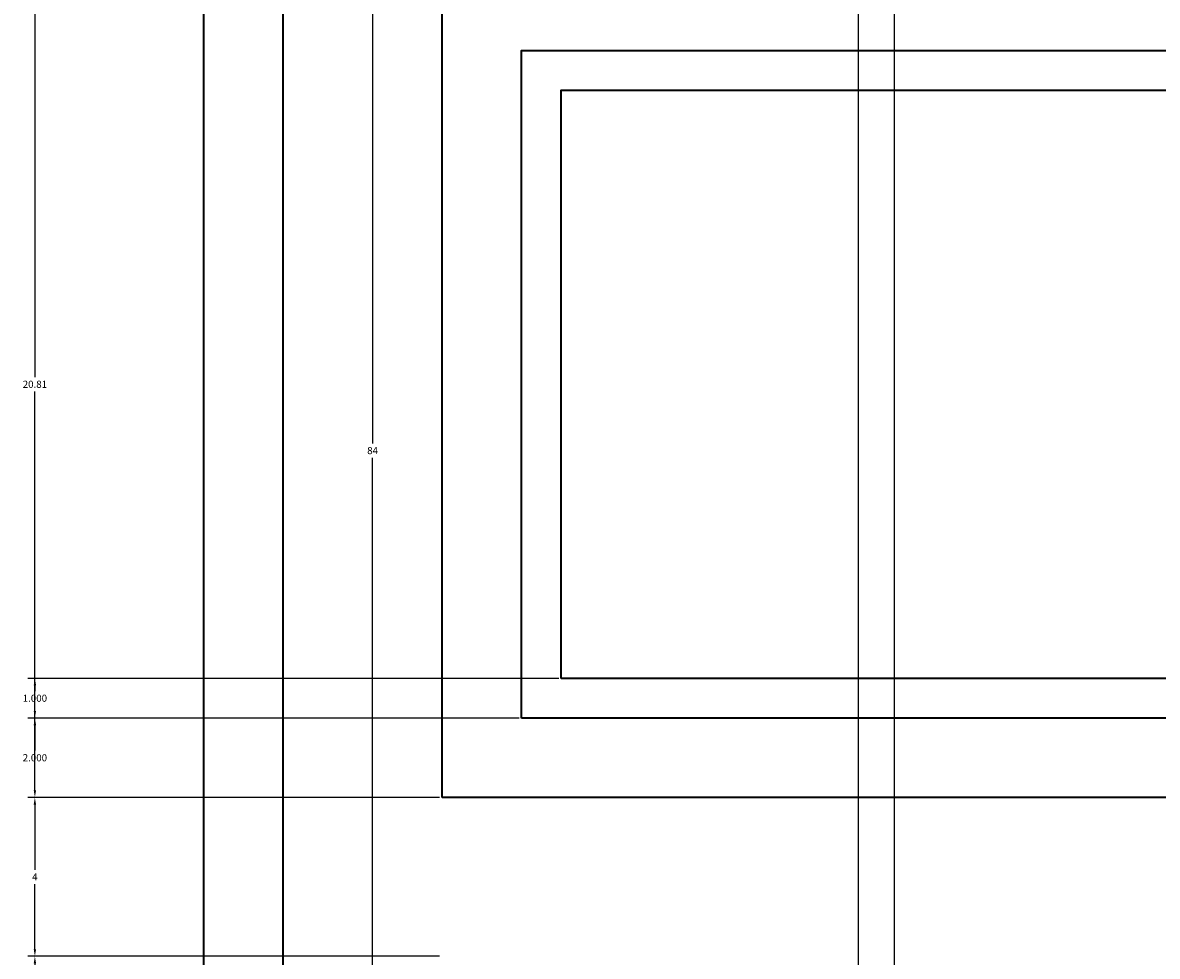
# Model space of a CAD drawing. Units: inches. Extents: x 3137 to 3299, y 1994 to 2089.
# Tile 3 of 14: x 3137 to 3165, y 2028 to 2052. Entities that reach past the tile are written whole.
import ezdxf

# ---------------------------------------------------------------- set-up
doc = ezdxf.new("R2010")
doc.units = ezdxf.units.IN
doc.header["$MEASUREMENT"] = 0
doc.layers.add('A-ANNO-DIMS', color=2, linetype='Continuous', lineweight=18)
doc.layers.add('A-DOOR', color=4, linetype='Continuous', lineweight=35)
doc.styles.get("Standard").update_dxf_attribs({"font": 'arial.ttf'})
doc.dimstyles.get("Standard").update_dxf_attribs({"dimtxt": 0.18, "dimasz": 0.18, "dimexe": 0.18, "dimexo": 0.0625, "dimgap": 0.09, "dimtad": 0, "dimtih": 1, "dimtoh": 1, "dimdec": 4, "dimzin": 0, "dimdsep": 46, "dimtxsty": 'Standard', "dimcen": 0.09, "dimadec": 0, "dimazin": 0, "dimtfac": 1, "dimtdec": 4, "dimtofl": 0, "dimtmove": 0, "dimatfit": 3, "dimfxl": 1, "dimtolj": 1, "dimtzin": 0, "dimarcsym": 0})

# ---------------------------------------------------------------- blocks, each defined once
blk = doc.blocks.new('*D40')
at = {"layer": 'A-ANNO-DIMS', "color": 0, "lineweight": -2, "transparency": 16777216}
for p, q in [((3147.415, 2028.138), (3137.048, 2028.138)), ((3137.228, 2027.958), (3137.228, 2027.318)), ((3137.228, 2026.318), (3137.228, 2026.957)), ((3149.415, 2026.138), (3137.048, 2026.138))]:
    blk.add_line(p, q, dxfattribs=at)
at = {"layer": 'A-ANNO-DIMS', "color": 0, "transparency": 16777216}
for points in [[(3137.198, 2027.958), (3137.258, 2027.958), (3137.228, 2028.138)], [(3137.198, 2026.318), (3137.258, 2026.318), (3137.228, 2026.138)]]:
    blk.add_solid(points, dxfattribs=at)
at = {"layer": 'Defpoints', "color": 0, "transparency": 16777216}
for p in [(3137.228, 2028.138), (3147.478, 2028.138), (3149.478, 2026.138)]:
    blk.add_point(p, dxfattribs=at)
at = {"layer": 'A-ANNO-DIMS', "color": 0, "transparency": 16777216, "insert": (3137.228, 2027.138), "char_height": 0.18, "attachment_point": 5}
blk.add_mtext('\\A1;2', dxfattribs=at)
blk = doc.blocks.new('*D41')
at = {"layer": 'A-ANNO-DIMS', "color": 0, "lineweight": -2, "transparency": 16777216}
for p, q in [((3147.415181, 2032.137537), (3137.047681, 2032.137537)), ((3137.227681, 2031.957537), (3137.227681, 2030.317537)), ((3137.227681, 2028.317537), (3137.227681, 2029.957537)), ((3147.415181, 2028.137537), (3137.047681, 2028.137537))]:
    blk.add_line(p, q, dxfattribs=at)
at = {"layer": 'A-ANNO-DIMS', "color": 0, "transparency": 16777216}
for points in [[(3137.197681, 2031.957537), (3137.257681, 2031.957537), (3137.227681, 2032.137537)], [(3137.197681, 2028.317537), (3137.257681, 2028.317537), (3137.227681, 2028.137537)]]:
    blk.add_solid(points, dxfattribs=at)
at = {"layer": 'Defpoints', "color": 0, "transparency": 16777216}
for p in [(3137.227681, 2032.137537), (3147.477681, 2032.137537), (3147.477681, 2028.137537)]:
    blk.add_point(p, dxfattribs=at)
at = {"layer": 'A-ANNO-DIMS', "color": 0, "transparency": 16777216, "insert": (3137.227681, 2030.137537), "char_height": 0.18, "attachment_point": 5}
blk.add_mtext('\\A1;4', dxfattribs=at)
blk = doc.blocks.new('*D42')
at = {"layer": 'A-ANNO-DIMS', "color": 0, "lineweight": -2, "transparency": 16777216}
for p, q in [((3147.415, 2052.948), (3137.048, 2052.948)), ((3137.228, 2052.768), (3137.228, 2042.725)), ((3137.228, 2032.318), (3137.228, 2042.361)), ((3147.415, 2032.138), (3137.048, 2032.138))]:
    blk.add_line(p, q, dxfattribs=at)
at = {"layer": 'A-ANNO-DIMS', "color": 0, "transparency": 16777216}
for points in [[(3137.198, 2052.768), (3137.258, 2052.768), (3137.228, 2052.948)], [(3137.198, 2032.318), (3137.258, 2032.318), (3137.228, 2032.138)]]:
    blk.add_solid(points, dxfattribs=at)
at = {"layer": 'Defpoints', "color": 0, "transparency": 16777216}
for p in [(3137.228, 2052.948), (3147.478, 2052.948), (3147.478, 2032.138)]:
    blk.add_point(p, dxfattribs=at)
at = {"layer": 'A-ANNO-DIMS', "color": 0, "transparency": 16777216, "insert": (3137.228, 2042.543), "char_height": 0.18, "attachment_point": 5}
blk.add_mtext('\\A1;20.81', dxfattribs=at)
blk = doc.blocks.new('*D55')
at = {"layer": 'A-ANNO-DIMS', "color": 0, "lineweight": -2, "transparency": 16777216}
for p, q in [((3141.54, 2082.874), (3145.908, 2082.874)), ((3145.728, 2082.694), (3145.728, 2041.056)), ((3145.728, 1999.054), (3145.728, 2040.692)), ((3141.54, 1998.874), (3145.908, 1998.874))]:
    blk.add_line(p, q, dxfattribs=at)
at = {"layer": 'A-ANNO-DIMS', "color": 0, "transparency": 16777216}
for points in [[(3145.698, 2082.694), (3145.758, 2082.694), (3145.728, 2082.874)], [(3145.698, 1999.054), (3145.758, 1999.054), (3145.728, 1998.874)]]:
    blk.add_solid(points, dxfattribs=at)
at = {"layer": 'Defpoints', "color": 0, "transparency": 16777216}
for p in [(3141.478, 2082.874), (3141.478, 1998.874), (3145.728, 1998.874)]:
    blk.add_point(p, dxfattribs=at)
at = {"layer": 'A-ANNO-DIMS', "color": 0, "transparency": 16777216, "insert": (3145.728, 2040.874), "char_height": 0.18, "attachment_point": 5}
blk.add_mtext('\\A1;84', dxfattribs=at)
blk = doc.blocks.new('*D77')
at = {"layer": 'A-ANNO-DIMS', "color": 0, "lineweight": -2, "transparency": 16777216}
for p, q in [((3149.415, 2034.138), (3137.048, 2034.138)), ((3137.228, 2033.958), (3137.228, 2033.319)), ((3137.228, 2032.318), (3137.228, 2032.956)), ((3147.415, 2032.138), (3137.048, 2032.138))]:
    blk.add_line(p, q, dxfattribs=at)
at = {"layer": 'A-ANNO-DIMS', "color": 0, "transparency": 16777216}
for points in [[(3137.198, 2033.958), (3137.258, 2033.958), (3137.228, 2034.138)], [(3137.198, 2032.318), (3137.258, 2032.318), (3137.228, 2032.138)]]:
    blk.add_solid(points, dxfattribs=at)
at = {"layer": 'Defpoints', "color": 0, "transparency": 16777216}
for p in [(3137.228, 2034.138), (3149.478, 2034.138), (3147.478, 2032.138)]:
    blk.add_point(p, dxfattribs=at)
at = {"layer": 'A-ANNO-DIMS', "color": 0, "transparency": 16777216, "insert": (3137.228, 2033.138), "char_height": 0.18, "attachment_point": 5}
blk.add_mtext('\\A1;2.000', dxfattribs=at)
blk = doc.blocks.new('*D78')
at = {"layer": 'A-ANNO-DIMS', "color": 0, "lineweight": -2, "transparency": 16777216}
for p, q in [((3150.415, 2035.138), (3137.048, 2035.138)), ((3137.228, 2034.958), (3137.228, 2034.819)), ((3137.228, 2034.318), (3137.228, 2034.456)), ((3149.415, 2034.138), (3137.048, 2034.138))]:
    blk.add_line(p, q, dxfattribs=at)
at = {"layer": 'A-ANNO-DIMS', "color": 0, "transparency": 16777216}
for points in [[(3137.198, 2034.958), (3137.258, 2034.958), (3137.228, 2035.138)], [(3137.198, 2034.318), (3137.258, 2034.318), (3137.228, 2034.138)]]:
    blk.add_solid(points, dxfattribs=at)
at = {"layer": 'Defpoints', "color": 0, "transparency": 16777216}
for p in [(3137.228, 2035.138), (3150.478, 2035.138), (3149.478, 2034.138)]:
    blk.add_point(p, dxfattribs=at)
at = {"layer": 'A-ANNO-DIMS', "color": 0, "transparency": 16777216, "insert": (3137.228, 2034.638), "char_height": 0.18, "attachment_point": 5}
blk.add_mtext('\\A1;1.000', dxfattribs=at)
blk = doc.blocks.new('*D81')
at = {"layer": 'A-ANNO-DIMS', "color": 0, "lineweight": -2, "transparency": 16777216}
for p, q in [((3157.951, 2066.849), (3157.951, 1994.444)), ((3158.858, 2065.44), (3158.858, 1994.444)), ((3157.771, 1994.624), (3157.591, 1994.624)), ((3159.038, 1994.624), (3159.218, 1994.624))]:
    blk.add_line(p, q, dxfattribs=at)
at = {"layer": 'A-ANNO-DIMS', "color": 0, "transparency": 16777216}
for points in [[(3157.771, 1994.654), (3157.771, 1994.594), (3157.951, 1994.624)], [(3159.038, 1994.654), (3159.038, 1994.594), (3158.858, 1994.624)]]:
    blk.add_solid(points, dxfattribs=at)
at = {"layer": 'Defpoints', "color": 0, "transparency": 16777216}
for p in [(3157.951, 2066.911), (3158.858, 2065.503), (3158.858, 1994.624)]:
    blk.add_point(p, dxfattribs=at)
at = {"layer": 'A-ANNO-DIMS', "color": 0, "transparency": 16777216, "insert": (3158.404, 1994.624), "char_height": 0.18, "attachment_point": 5}
blk.add_mtext('\\A1;0.907', dxfattribs=at)

msp = doc.modelspace()

# ---------------------------------------------------------------- linework, layer by layer
at = {"layer": 'A-DOOR'}
for points in [[(3141.4777, 2082.874), (3189.4777, 2082.874), (3189.4777, 1998.874), (3141.4777, 1998.874)], [(3147.4777, 2032.1375), (3147.4777, 2052.9483), (3183.4777, 2052.9483), (3183.4777, 2032.1375)], [(3149.4777, 2034.1375), (3149.4777, 2050.9483), (3181.4777, 2050.9483), (3181.4777, 2034.1375)], [(3150.4777, 2035.1375), (3150.4777, 2049.9483), (3180.4777, 2049.9483), (3180.4777, 2035.1375)]]:
    msp.add_lwpolyline(points, close=True, dxfattribs=at)
msp.add_lwpolyline([(3187.4777, 2007.6773), (3187.4777, 2000.874), (3143.4777, 2000.874), (3143.4777, 2080.874), (3187.4777, 2080.874), (3187.4777, 2076.298)], dxfattribs=at)

# ---------------------------------------------------------------- dimensions: what is measured, and where the dimension line sits
at = {"layer": 'A-ANNO-DIMS'}
for base, p1, p2, angle, override, picture, middle in [((3145.7277, 1998.874), (3141.4777, 2082.874), (3141.4777, 1998.874), 270, {"dimdec": 0, "dimlfac": 1, "dimrnd": 0, "dimzin": 0, "dimdsep": 46, "dimlunit": 2}, '*D55', (3145.7277, 2040.874)), ((3137.2277, 2052.9483), (3147.4777, 2032.1375), (3147.4777, 2052.9483), 90, {"dimdec": 2, "dimlfac": 1, "dimrnd": 0, "dimzin": 0, "dimdsep": 46, "dimlunit": 2}, '*D42', (3137.2277, 2042.5429)), ((3137.2277, 2035.1375), (3149.4777, 2034.1375), (3150.4777, 2035.1375), 90, {"dimdec": 3, "dimlfac": 1, "dimrnd": 0, "dimzin": 0, "dimdsep": 46, "dimlunit": 2}, '*D78', (3137.2277, 2034.6375)), ((3137.2277, 2034.1375), (3147.4777, 2032.1375), (3149.4777, 2034.1375), 90, {"dimdec": 3, "dimlfac": 1, "dimrnd": 0, "dimzin": 0, "dimdsep": 46, "dimlunit": 2}, '*D77', (3137.2277, 2033.1375)), ((3137.2277, 2032.1375), (3147.4777, 2028.1375), (3147.4777, 2032.1375), 90, {"dimdec": 0, "dimlfac": 1, "dimrnd": 0, "dimzin": 0, "dimdsep": 46, "dimlunit": 2}, '*D41', (3137.2277, 2030.1375)), ((3137.2277, 2028.1375), (3149.4777, 2026.1375), (3147.4777, 2028.1375), 90, {"dimdec": 0, "dimlfac": 1, "dimrnd": 0, "dimzin": 0, "dimdsep": 46, "dimlunit": 2}, '*D40', (3137.2277, 2027.1375))]:
    dim = msp.add_linear_dim(base=base, p1=p1, p2=p2, angle=angle, dimstyle='Standard', override=override, dxfattribs=at)
    dim.commit()
    dim.dimension.update_dxf_attribs({"geometry": picture, "text_midpoint": middle})
dim = msp.add_linear_dim(base=(3158.8577, 1994.624), p1=(3157.9507, 2066.9111), p2=(3158.8577, 2065.5029), dimstyle='Standard', override={"dimdec": 3, "dimlfac": 1, "dimrnd": 0, "dimzin": 0, "dimdsep": 46, "dimlunit": 2}, dxfattribs=at)
dim.commit()
dim.dimension.update_dxf_attribs({"geometry": '*D81', "text_midpoint": (3158.4042, 1994.624)})

doc.saveas('drawing.dxf')
